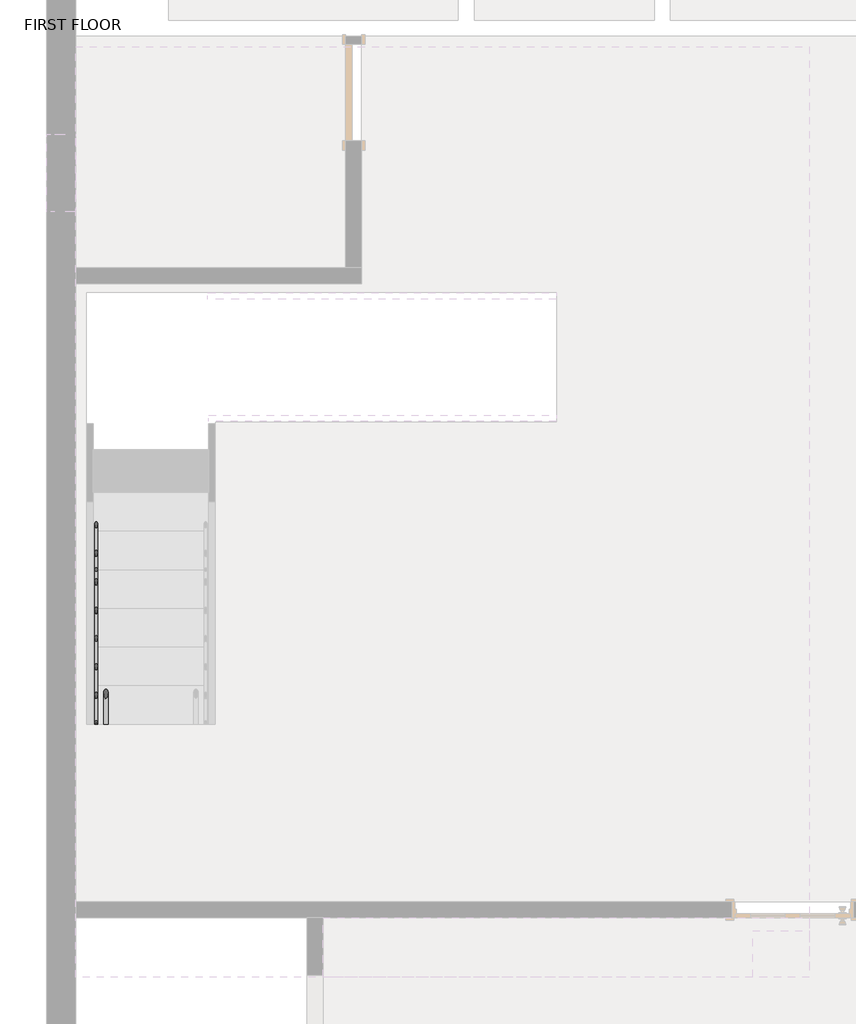
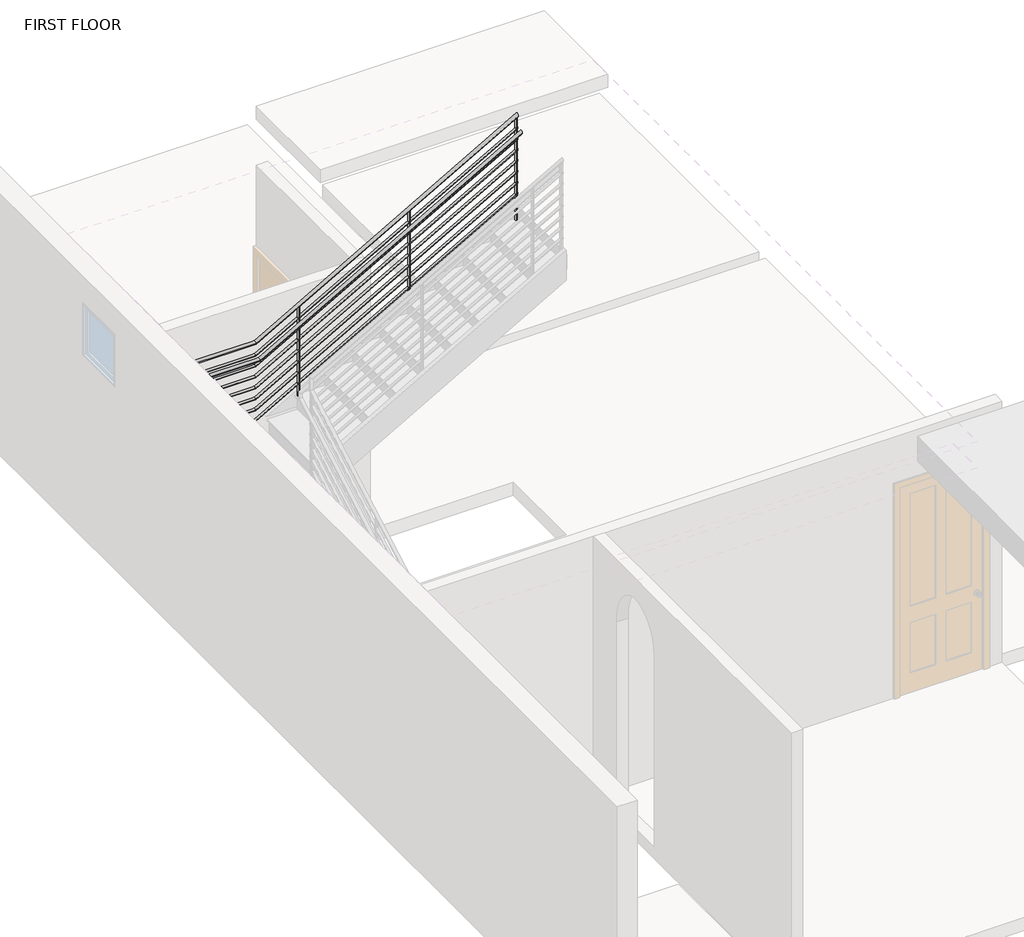
# One storey, part 2 of 3: 1 railing.
"""IFC4 building model written with IfcOpenShell, lengths in millimetres."""

from ifc_helpers import new_model, si_unit, point, frame, frame_2d, origin, place, context, project, spatial, circle_curve, ellipse_curve, trimmed, segment, composite_curve, outline, extrude, element, save
from ifc_brep_helpers import plane_surface, cylinder_surface, advanced_brep

model = new_model("IFC4")

# Units and contexts
model_context = context("Model", 3, world=origin())
ifc_project = project(units=[si_unit("LENGTHUNIT", "METRE", prefix="MILLI")], contexts=[model_context])

# Site, building, storey
site = spatial("IfcSite", under=ifc_project)
building = spatial("IfcBuilding", under=site)
storey = spatial("IfcBuildingStorey", under=building, Name="FIRST FLOOR", Elevation=3352.8)

# Railing
placement = place(None, origin())
element("IfcRailing", 1, ObjectType="Guardrail - Pipe", at=placement, inside=storey, context=model_context, shape_type="SolidModel", body=[
    advanced_brep(
    [(-6821.0257327, 1771.427543, 4418.0240066), (-6859.1257327, 1771.427543, 4418.0240066), (-6821.0257327, 4367.2498842, 5888.99), (-6859.1257327, 4367.2498842, 5888.99), (-6821.0257327, 5003.577543, 5888.99), (-6859.1257327, 5041.677543, 5888.99), (-6174.6533915, 5003.577543, 5888.99), (-6174.6533915, 5041.677543, 5888.99), (-3284.0757327, 5003.577543, 7526.9840066), (-3284.0757327, 5041.677543, 7526.9840066)],
    [
        (0, 1, ellipse_curve(frame((-6840.0757327, 1771.427543, 4418.0240066), z_axis=(0.0, -1.0, 0.0), x_axis=(0.0, 0.0, -1.0)), 21.8959934, 19.05)),
        (1, 0, ellipse_curve(frame((-6840.0757327, 1771.427543, 4418.0240066), z_axis=(0.0, -1.0, 0.0), x_axis=(0.0, 0.0, -1.0)), 21.8959934, 19.05)),
        (0, 2),
        (2, 3, ellipse_curve(frame((-6840.0757327, 4367.2498842, 5888.99), z_axis=(0.0, -0.9669597162882765, -0.25492921973696103), x_axis=(0.0, 0.25492921973696087, -0.9669597162882766)), 19.7009241, 19.05)),
        (3, 1),
        (3, 2, ellipse_curve(frame((-6840.0757327, 4367.2498842, 5888.99), z_axis=(0.0, -0.9669597162882765, -0.25492921973696103), x_axis=(0.0, 0.25492921973696087, -0.9669597162882766)), 19.7009241, 19.05)),
        (2, 4),
        (4, 5, ellipse_curve(frame((-6840.0757327, 5022.627543, 5888.99), z_axis=(-0.7071067811865486, -0.7071067811865465, 0.0), x_axis=(0.7071067811865465, -0.7071067811865486, 0.0)), 26.9407684, 19.05)),
        (5, 3),
        (5, 4, ellipse_curve(frame((-6840.0757327, 5022.627543, 5888.99), z_axis=(-0.7071067811865486, -0.7071067811865465, 0.0), x_axis=(0.7071067811865465, -0.7071067811865486, 0.0)), 26.9407684, 19.05)),
        (4, 6),
        (6, 7, ellipse_curve(frame((-6174.6533915, 5022.627543, 5888.99), z_axis=(-0.9669597162882765, 0.0, -0.254929219736961), x_axis=(-0.25492921973696137, 0.0, 0.9669597162882764)), 19.7009241, 19.05)),
        (7, 5),
        (7, 6, ellipse_curve(frame((-6174.6533915, 5022.627543, 5888.99), z_axis=(-0.9669597162882765, 0.0, -0.254929219736961), x_axis=(-0.25492921973696137, 0.0, 0.9669597162882764)), 19.7009241, 19.05)),
        (8, 9, ellipse_curve(frame((-3284.0757327, 5022.627543, 7526.9840066), z_axis=(1.0, 0.0, 0.0), x_axis=(0.0, 0.0, -0.9999999999999999)), 21.8959934, 19.05)),
        (9, 8, ellipse_curve(frame((-3284.0757327, 5022.627543, 7526.9840066), z_axis=(1.0, 0.0, 0.0), x_axis=(0.0, 0.0, -0.9999999999999999)), 21.8959934, 19.05)),
        (6, 8),
        (9, 7),
    ],
    [
        plane_surface(frame((-6840.0757327, 1771.427543, 4439.92), z_axis=(0.0, -1.0, 0.0), x_axis=(0.0, 0.0, 1.0))),
        cylinder_surface(frame((-6840.0757327, 1780.8194325, 4423.3460774), z_axis=(0.0, -0.8700221858486086, -0.4930125719808871), x_axis=(-1.0, 0.0, 0.0)), 19.05),
        cylinder_surface(frame((-6840.0757327, 4362.227543, 5888.99), z_axis=(0.0, -1.0, 0.0), x_axis=(-1.0, 0.0, 0.0)), 19.05),
        cylinder_surface(frame((-6840.0757327, 5022.627543, 5888.99), z_axis=(-1.0, 0.0, 0.0), x_axis=(0.0, 1.0, 0.0)), 19.05),
        plane_surface(frame((-3284.0757327, 5022.627543, 7548.88), z_axis=(1.0, 0.0, 0.0), x_axis=(0.0, 1.0, 0.0))),
        cylinder_surface(frame((-6170.2838432, 5022.627543, 5891.4660774), z_axis=(-0.8700221858486086, 0.0, -0.49301257198088694), x_axis=(0.0, 1.0, 0.0)), 19.05),
    ],
    [
        (0, [[1, 2]]),
        (1, [[-1, 3, 4, 5]]),
        (1, [[-2, -5, 6, -3]]),
        (2, [[-4, 7, 8, 9]]),
        (2, [[-6, -9, 10, -7]]),
        (3, [[-8, 11, 12, 13]]),
        (3, [[-10, -13, 14, -11]]),
        (4, [[15, 16]]),
        (5, [[-12, 17, -16, 18]]),
        (5, [[-14, -18, -15, -17]]),
    ],
),
    advanced_brep(
    [(-6897.2257327, 1771.427543, 4570.4240066), (-6935.3257327, 1771.427543, 4570.4240066), (-3284.0757327, 5079.777543, 7679.3840066), (-3284.0757327, 5117.877543, 7679.3840066), (-6897.2257327, 4367.2498842, 6041.39), (-6935.3257327, 4367.2498842, 6041.39), (-6897.2257327, 5079.777543, 6041.39), (-6935.3257327, 5117.877543, 6041.39), (-6174.6533915, 5079.777543, 6041.39), (-6174.6533915, 5117.877543, 6041.39)],
    [
        (0, 1, ellipse_curve(frame((-6916.2757327, 1771.427543, 4570.4240066), z_axis=(0.0, -1.0, 0.0), x_axis=(0.0, 0.0, -1.0)), 21.8959934, 19.05)),
        (1, 0, ellipse_curve(frame((-6916.2757327, 1771.427543, 4570.4240066), z_axis=(0.0, -1.0, 0.0), x_axis=(0.0, 0.0, -1.0)), 21.8959934, 19.05)),
        (2, 3, ellipse_curve(frame((-3284.0757327, 5098.827543, 7679.3840066), z_axis=(1.0, 0.0, 0.0), x_axis=(0.0, 0.0, -0.9999999999999999)), 21.8959934, 19.05)),
        (3, 2, ellipse_curve(frame((-3284.0757327, 5098.827543, 7679.3840066), z_axis=(1.0, 0.0, 0.0), x_axis=(0.0, 0.0, -0.9999999999999999)), 21.8959934, 19.05)),
        (0, 4),
        (4, 5, ellipse_curve(frame((-6916.2757327, 4367.2498842, 6041.39), z_axis=(0.0, -0.9669597162882765, -0.25492921973696103), x_axis=(0.0, 0.25492921973696087, -0.9669597162882766)), 19.7009241, 19.05)),
        (5, 1),
        (5, 4, ellipse_curve(frame((-6916.2757327, 4367.2498842, 6041.39), z_axis=(0.0, -0.9669597162882765, -0.25492921973696103), x_axis=(0.0, 0.25492921973696087, -0.9669597162882766)), 19.7009241, 19.05)),
        (4, 6),
        (6, 7, ellipse_curve(frame((-6916.2757327, 5098.827543, 6041.39), z_axis=(-0.7071067811865487, -0.7071067811865464, 0.0), x_axis=(0.7071067811865464, -0.7071067811865487, 0.0)), 26.9407684, 19.05)),
        (7, 5),
        (7, 6, ellipse_curve(frame((-6916.2757327, 5098.827543, 6041.39), z_axis=(-0.7071067811865487, -0.7071067811865464, 0.0), x_axis=(0.7071067811865464, -0.7071067811865487, 0.0)), 26.9407684, 19.05)),
        (6, 8),
        (8, 9, ellipse_curve(frame((-6174.6533915, 5098.827543, 6041.39), z_axis=(-0.9669597162882765, 0.0, -0.254929219736961), x_axis=(-0.25492921973696137, 0.0, 0.9669597162882764)), 19.7009241, 19.05)),
        (9, 7),
        (9, 8, ellipse_curve(frame((-6174.6533915, 5098.827543, 6041.39), z_axis=(-0.9669597162882765, 0.0, -0.254929219736961), x_axis=(-0.25492921973696137, 0.0, 0.9669597162882764)), 19.7009241, 19.05)),
        (8, 2),
        (3, 9),
    ],
    [
        plane_surface(frame((-6916.2757327, 1771.427543, 4592.32), z_axis=(0.0, -1.0, 0.0), x_axis=(0.0, 0.0, 1.0))),
        plane_surface(frame((-3284.0757327, 5098.827543, 7701.28), z_axis=(1.0, 0.0, 0.0), x_axis=(0.0, 1.0, 0.0))),
        cylinder_surface(frame((-6916.2757327, 1780.8194325, 4575.7460774), z_axis=(0.0, -0.8700221858486086, -0.4930125719808871), x_axis=(-1.0, 0.0, 0.0)), 19.05),
        cylinder_surface(frame((-6916.2757327, 4362.227543, 6041.39), z_axis=(0.0, -1.0, 0.0), x_axis=(-1.0, 0.0, 0.0)), 19.05),
        cylinder_surface(frame((-6916.2757327, 5098.827543, 6041.39), z_axis=(-1.0, 0.0, 0.0), x_axis=(0.0, 1.0, 0.0)), 19.05),
        cylinder_surface(frame((-6170.2838432, 5098.827543, 6043.8660774), z_axis=(-0.8700221858486086, 0.0, -0.49301257198088694), x_axis=(0.0, 1.0, 0.0)), 19.05),
    ],
    [
        (0, [[1, 2]]),
        (1, [[3, 4]]),
        (2, [[-1, 5, 6, 7]]),
        (2, [[-2, -7, 8, -5]]),
        (3, [[-6, 9, 10, 11]]),
        (3, [[-8, -11, 12, -9]]),
        (4, [[-10, 13, 14, 15]]),
        (4, [[-12, -15, 16, -13]]),
        (5, [[-14, 17, -4, 18]]),
        (5, [[-16, -18, -3, -17]]),
    ],
),
    advanced_brep(
    [(-6903.5757327, 1771.427543, 4425.3226711), (-6928.9757327, 1771.427543, 4425.3226711), (-6903.5757327, 4365.5757705, 5895.34), (-6928.9757327, 4365.5757705, 5895.34), (-6903.5757327, 5086.127543, 5895.34), (-6928.9757327, 5086.127543, 5895.34)],
    [
        (0, 1, ellipse_curve(frame((-6916.2757327, 1771.427543, 4425.3226711), z_axis=(0.0, -1.0, 0.0), x_axis=(0.0, 0.0, -1.0)), 14.5973289, 12.7)),
        (1, 0, ellipse_curve(frame((-6916.2757327, 1771.427543, 4425.3226711), z_axis=(0.0, -1.0, 0.0), x_axis=(0.0, 0.0, -1.0)), 14.5973289, 12.7)),
        (0, 2),
        (2, 3, ellipse_curve(frame((-6916.2757327, 4365.5757705, 5895.34), z_axis=(0.0, -0.9669597162882765, -0.25492921973696103), x_axis=(0.0, 0.25492921973696087, -0.9669597162882766)), 13.1339494, 12.7)),
        (3, 1),
        (3, 2, ellipse_curve(frame((-6916.2757327, 4365.5757705, 5895.34), z_axis=(0.0, -0.9669597162882765, -0.25492921973696103), x_axis=(0.0, 0.25492921973696087, -0.9669597162882766)), 13.1339494, 12.7)),
        (4, 5, circle_curve(frame((-6916.2757327, 5086.127543, 5895.34), z_axis=(0.0, 1.0, 0.0), x_axis=(-1.0, 0.0, 0.0)), 12.7)),
        (5, 4, circle_curve(frame((-6916.2757327, 5086.127543, 5895.34), z_axis=(0.0, 1.0, 0.0), x_axis=(-1.0, 0.0, 0.0)), 12.7)),
        (2, 4),
        (5, 3),
    ],
    [
        plane_surface(frame((-6916.2757327, 1771.427543, 4439.92), z_axis=(0.0, -1.0, 0.0), x_axis=(0.0, 0.0, 1.0))),
        cylinder_surface(frame((-6916.2757327, 1777.6888026, 4428.8707182), z_axis=(0.0, -0.8700221858486086, -0.4930125719808871), x_axis=(-1.0, 0.0, 0.0)), 12.7),
        plane_surface(frame((-6916.2757327, 5086.127543, 5908.04), z_axis=(0.0, 1.0, 0.0), x_axis=(0.0, 0.0, 1.0))),
        cylinder_surface(frame((-6916.2757327, 4362.227543, 5895.34), z_axis=(0.0, -1.0, 0.0), x_axis=(-1.0, 0.0, 0.0)), 12.7),
    ],
    [
        (0, [[1, 2]]),
        (1, [[-1, 3, 4, 5]]),
        (1, [[-2, -5, 6, -3]]),
        (2, [[7, 8]]),
        (3, [[-4, 9, -8, 10]]),
        (3, [[-6, -10, -7, -9]]),
    ],
),
    advanced_brep(
    [(-6928.9757327, 5086.127543, 5895.34), (-6928.9757327, 5111.527543, 5895.34), (-6176.3275052, 5086.127543, 5895.34), (-6176.3275052, 5111.527543, 5895.34), (-3284.0757327, 5086.127543, 7534.2826711), (-3284.0757327, 5111.527543, 7534.2826711)],
    [
        (0, 1, circle_curve(frame((-6928.9757327, 5098.827543, 5895.34), z_axis=(-1.0, 0.0, 0.0), x_axis=(0.0, 1.0, 0.0)), 12.7)),
        (1, 0, circle_curve(frame((-6928.9757327, 5098.827543, 5895.34), z_axis=(-1.0, 0.0, 0.0), x_axis=(0.0, 1.0, 0.0)), 12.7)),
        (0, 2),
        (2, 3, ellipse_curve(frame((-6176.3275052, 5098.827543, 5895.34), z_axis=(-0.9669597162882765, 0.0, -0.2549292197369609), x_axis=(-0.25492921973696137, 0.0, 0.9669597162882764)), 13.1339494, 12.7)),
        (3, 1),
        (3, 2, ellipse_curve(frame((-6176.3275052, 5098.827543, 5895.34), z_axis=(-0.9669597162882765, 0.0, -0.2549292197369609), x_axis=(-0.25492921973696137, 0.0, 0.9669597162882764)), 13.1339494, 12.7)),
        (4, 5, ellipse_curve(frame((-3284.0757327, 5098.827543, 7534.2826711), z_axis=(1.0, 0.0, 0.0), x_axis=(0.0, 0.0, -0.9999999999999999)), 14.5973289, 12.7)),
        (5, 4, ellipse_curve(frame((-3284.0757327, 5098.827543, 7534.2826711), z_axis=(1.0, 0.0, 0.0), x_axis=(0.0, 0.0, -0.9999999999999999)), 14.5973289, 12.7)),
        (2, 4),
        (5, 3),
    ],
    [
        plane_surface(frame((-6928.9757327, 5098.827543, 5908.04), z_axis=(-1.0, 0.0, 0.0), x_axis=(0.0, 1.0, 0.0))),
        cylinder_surface(frame((-6928.9757327, 5098.827543, 5895.34), z_axis=(-1.0, 0.0, 0.0), x_axis=(0.0, 1.0, 0.0)), 12.7),
        plane_surface(frame((-3284.0757327, 5098.827543, 7548.88), z_axis=(1.0, 0.0, 0.0), x_axis=(0.0, 1.0, 0.0))),
        cylinder_surface(frame((-6173.414473, 5098.827543, 5896.9907182), z_axis=(-0.8700221858486087, 0.0, -0.49301257198088694), x_axis=(0.0, 1.0, 0.0)), 12.7),
    ],
    [
        (0, [[1, 2]]),
        (1, [[-1, 3, 4, 5]]),
        (1, [[-2, -5, 6, -3]]),
        (2, [[7, 8]]),
        (3, [[-4, 9, -8, 10]]),
        (3, [[-6, -10, -7, -9]]),
    ],
),
    advanced_brep(
    [(-6903.5757327, 1771.427543, 4298.3226711), (-6928.9757327, 1771.427543, 4298.3226711), (-6903.5757327, 4365.5757705, 5768.34), (-6928.9757327, 4365.5757705, 5768.34), (-6903.5757327, 5086.127543, 5768.34), (-6928.9757327, 5086.127543, 5768.34)],
    [
        (0, 1, ellipse_curve(frame((-6916.2757327, 1771.427543, 4298.3226711), z_axis=(0.0, -1.0, 0.0), x_axis=(0.0, 0.0, -1.0)), 14.5973289, 12.7)),
        (1, 0, ellipse_curve(frame((-6916.2757327, 1771.427543, 4298.3226711), z_axis=(0.0, -1.0, 0.0), x_axis=(0.0, 0.0, -1.0)), 14.5973289, 12.7)),
        (0, 2),
        (2, 3, ellipse_curve(frame((-6916.2757327, 4365.5757705, 5768.34), z_axis=(0.0, -0.9669597162882765, -0.25492921973696103), x_axis=(0.0, 0.25492921973696087, -0.9669597162882766)), 13.1339494, 12.7)),
        (3, 1),
        (3, 2, ellipse_curve(frame((-6916.2757327, 4365.5757705, 5768.34), z_axis=(0.0, -0.9669597162882765, -0.25492921973696103), x_axis=(0.0, 0.25492921973696087, -0.9669597162882766)), 13.1339494, 12.7)),
        (4, 5, circle_curve(frame((-6916.2757327, 5086.127543, 5768.34), z_axis=(0.0, 1.0, 0.0), x_axis=(-1.0, 0.0, 0.0)), 12.7)),
        (5, 4, circle_curve(frame((-6916.2757327, 5086.127543, 5768.34), z_axis=(0.0, 1.0, 0.0), x_axis=(-1.0, 0.0, 0.0)), 12.7)),
        (2, 4),
        (5, 3),
    ],
    [
        plane_surface(frame((-6916.2757327, 1771.427543, 4312.92), z_axis=(0.0, -1.0, 0.0), x_axis=(0.0, 0.0, 1.0))),
        cylinder_surface(frame((-6916.2757327, 1777.6888026, 4301.8707182), z_axis=(0.0, -0.8700221858486086, -0.4930125719808871), x_axis=(-1.0, 0.0, 0.0)), 12.7),
        plane_surface(frame((-6916.2757327, 5086.127543, 5781.04), z_axis=(0.0, 1.0, 0.0), x_axis=(0.0, 0.0, 1.0))),
        cylinder_surface(frame((-6916.2757327, 4362.227543, 5768.34), z_axis=(0.0, -1.0, 0.0), x_axis=(-1.0, 0.0, 0.0)), 12.7),
    ],
    [
        (0, [[1, 2]]),
        (1, [[-1, 3, 4, 5]]),
        (1, [[-2, -5, 6, -3]]),
        (2, [[7, 8]]),
        (3, [[-4, 9, -8, 10]]),
        (3, [[-6, -10, -7, -9]]),
    ],
),
    advanced_brep(
    [(-6928.9757327, 5086.127543, 5768.34), (-6928.9757327, 5111.527543, 5768.34), (-6176.3275052, 5086.127543, 5768.34), (-6176.3275052, 5111.527543, 5768.34), (-3284.0757327, 5086.127543, 7407.2826711), (-3284.0757327, 5111.527543, 7407.2826711)],
    [
        (0, 1, circle_curve(frame((-6928.9757327, 5098.827543, 5768.34), z_axis=(-1.0, 0.0, 0.0), x_axis=(0.0, 1.0, 0.0)), 12.7)),
        (1, 0, circle_curve(frame((-6928.9757327, 5098.827543, 5768.34), z_axis=(-1.0, 0.0, 0.0), x_axis=(0.0, 1.0, 0.0)), 12.7)),
        (0, 2),
        (2, 3, ellipse_curve(frame((-6176.3275052, 5098.827543, 5768.34), z_axis=(-0.9669597162882765, 0.0, -0.2549292197369609), x_axis=(-0.25492921973696137, 0.0, 0.9669597162882764)), 13.1339494, 12.7)),
        (3, 1),
        (3, 2, ellipse_curve(frame((-6176.3275052, 5098.827543, 5768.34), z_axis=(-0.9669597162882765, 0.0, -0.2549292197369609), x_axis=(-0.25492921973696137, 0.0, 0.9669597162882764)), 13.1339494, 12.7)),
        (4, 5, ellipse_curve(frame((-3284.0757327, 5098.827543, 7407.2826711), z_axis=(1.0, 0.0, 0.0), x_axis=(0.0, 0.0, -0.9999999999999999)), 14.5973289, 12.7)),
        (5, 4, ellipse_curve(frame((-3284.0757327, 5098.827543, 7407.2826711), z_axis=(1.0, 0.0, 0.0), x_axis=(0.0, 0.0, -0.9999999999999999)), 14.5973289, 12.7)),
        (2, 4),
        (5, 3),
    ],
    [
        plane_surface(frame((-6928.9757327, 5098.827543, 5781.04), z_axis=(-1.0, 0.0, 0.0), x_axis=(0.0, 1.0, 0.0))),
        cylinder_surface(frame((-6928.9757327, 5098.827543, 5768.34), z_axis=(-1.0, 0.0, 0.0), x_axis=(0.0, 1.0, 0.0)), 12.7),
        plane_surface(frame((-3284.0757327, 5098.827543, 7421.88), z_axis=(1.0, 0.0, 0.0), x_axis=(0.0, 1.0, 0.0))),
        cylinder_surface(frame((-6173.414473, 5098.827543, 5769.9907182), z_axis=(-0.8700221858486087, 0.0, -0.49301257198088694), x_axis=(0.0, 1.0, 0.0)), 12.7),
    ],
    [
        (0, [[1, 2]]),
        (1, [[-1, 3, 4, 5]]),
        (1, [[-2, -5, 6, -3]]),
        (2, [[7, 8]]),
        (3, [[-4, 9, -8, 10]]),
        (3, [[-6, -10, -7, -9]]),
    ],
),
    advanced_brep(
    [(-6903.5757327, 1771.427543, 4171.3226711), (-6928.9757327, 1771.427543, 4171.3226711), (-6903.5757327, 4365.5757705, 5641.34), (-6928.9757327, 4365.5757705, 5641.34), (-6903.5757327, 5086.127543, 5641.34), (-6928.9757327, 5086.127543, 5641.34)],
    [
        (0, 1, ellipse_curve(frame((-6916.2757327, 1771.427543, 4171.3226711), z_axis=(0.0, -1.0, 0.0), x_axis=(0.0, 0.0, -1.0)), 14.5973289, 12.7)),
        (1, 0, ellipse_curve(frame((-6916.2757327, 1771.427543, 4171.3226711), z_axis=(0.0, -1.0, 0.0), x_axis=(0.0, 0.0, -1.0)), 14.5973289, 12.7)),
        (0, 2),
        (2, 3, ellipse_curve(frame((-6916.2757327, 4365.5757705, 5641.34), z_axis=(0.0, -0.9669597162882765, -0.25492921973696103), x_axis=(0.0, 0.25492921973696087, -0.9669597162882766)), 13.1339494, 12.7)),
        (3, 1),
        (3, 2, ellipse_curve(frame((-6916.2757327, 4365.5757705, 5641.34), z_axis=(0.0, -0.9669597162882765, -0.25492921973696103), x_axis=(0.0, 0.25492921973696087, -0.9669597162882766)), 13.1339494, 12.7)),
        (4, 5, circle_curve(frame((-6916.2757327, 5086.127543, 5641.34), z_axis=(0.0, 1.0, 0.0), x_axis=(-1.0, 0.0, 0.0)), 12.7)),
        (5, 4, circle_curve(frame((-6916.2757327, 5086.127543, 5641.34), z_axis=(0.0, 1.0, 0.0), x_axis=(-1.0, 0.0, 0.0)), 12.7)),
        (2, 4),
        (5, 3),
    ],
    [
        plane_surface(frame((-6916.2757327, 1771.427543, 4185.92), z_axis=(0.0, -1.0, 0.0), x_axis=(0.0, 0.0, 1.0))),
        cylinder_surface(frame((-6916.2757327, 1777.6888026, 4174.8707182), z_axis=(0.0, -0.8700221858486086, -0.4930125719808871), x_axis=(-1.0, 0.0, 0.0)), 12.7),
        plane_surface(frame((-6916.2757327, 5086.127543, 5654.04), z_axis=(0.0, 1.0, 0.0), x_axis=(0.0, 0.0, 1.0))),
        cylinder_surface(frame((-6916.2757327, 4362.227543, 5641.34), z_axis=(0.0, -1.0, 0.0), x_axis=(-1.0, 0.0, 0.0)), 12.7),
    ],
    [
        (0, [[1, 2]]),
        (1, [[-1, 3, 4, 5]]),
        (1, [[-2, -5, 6, -3]]),
        (2, [[7, 8]]),
        (3, [[-4, 9, -8, 10]]),
        (3, [[-6, -10, -7, -9]]),
    ],
),
    advanced_brep(
    [(-6928.9757327, 5086.127543, 5641.34), (-6928.9757327, 5111.527543, 5641.34), (-6176.3275052, 5086.127543, 5641.34), (-6176.3275052, 5111.527543, 5641.34), (-3284.0757327, 5086.127543, 7280.2826711), (-3284.0757327, 5111.527543, 7280.2826711)],
    [
        (0, 1, circle_curve(frame((-6928.9757327, 5098.827543, 5641.34), z_axis=(-1.0, 0.0, 0.0), x_axis=(0.0, 1.0, 0.0)), 12.7)),
        (1, 0, circle_curve(frame((-6928.9757327, 5098.827543, 5641.34), z_axis=(-1.0, 0.0, 0.0), x_axis=(0.0, 1.0, 0.0)), 12.7)),
        (0, 2),
        (2, 3, ellipse_curve(frame((-6176.3275052, 5098.827543, 5641.34), z_axis=(-0.9669597162882765, 0.0, -0.2549292197369609), x_axis=(-0.25492921973696137, 0.0, 0.9669597162882764)), 13.1339494, 12.7)),
        (3, 1),
        (3, 2, ellipse_curve(frame((-6176.3275052, 5098.827543, 5641.34), z_axis=(-0.9669597162882765, 0.0, -0.2549292197369609), x_axis=(-0.25492921973696137, 0.0, 0.9669597162882764)), 13.1339494, 12.7)),
        (4, 5, ellipse_curve(frame((-3284.0757327, 5098.827543, 7280.2826711), z_axis=(1.0, 0.0, 0.0), x_axis=(0.0, 0.0, -0.9999999999999999)), 14.5973289, 12.7)),
        (5, 4, ellipse_curve(frame((-3284.0757327, 5098.827543, 7280.2826711), z_axis=(1.0, 0.0, 0.0), x_axis=(0.0, 0.0, -0.9999999999999999)), 14.5973289, 12.7)),
        (2, 4),
        (5, 3),
    ],
    [
        plane_surface(frame((-6928.9757327, 5098.827543, 5654.04), z_axis=(-1.0, 0.0, 0.0), x_axis=(0.0, 1.0, 0.0))),
        cylinder_surface(frame((-6928.9757327, 5098.827543, 5641.34), z_axis=(-1.0, 0.0, 0.0), x_axis=(0.0, 1.0, 0.0)), 12.7),
        plane_surface(frame((-3284.0757327, 5098.827543, 7294.88), z_axis=(1.0, 0.0, 0.0), x_axis=(0.0, 1.0, 0.0))),
        cylinder_surface(frame((-6173.414473, 5098.827543, 5642.9907182), z_axis=(-0.8700221858486087, 0.0, -0.49301257198088694), x_axis=(0.0, 1.0, 0.0)), 12.7),
    ],
    [
        (0, [[1, 2]]),
        (1, [[-1, 3, 4, 5]]),
        (1, [[-2, -5, 6, -3]]),
        (2, [[7, 8]]),
        (3, [[-4, 9, -8, 10]]),
        (3, [[-6, -10, -7, -9]]),
    ],
),
    advanced_brep(
    [(-6903.5757327, 1771.427543, 4044.3226711), (-6928.9757327, 1771.427543, 4044.3226711), (-6903.5757327, 4365.5757705, 5514.34), (-6928.9757327, 4365.5757705, 5514.34), (-6903.5757327, 5086.127543, 5514.34), (-6928.9757327, 5086.127543, 5514.34)],
    [
        (0, 1, ellipse_curve(frame((-6916.2757327, 1771.427543, 4044.3226711), z_axis=(0.0, -1.0, 0.0), x_axis=(0.0, 0.0, -1.0)), 14.5973289, 12.7)),
        (1, 0, ellipse_curve(frame((-6916.2757327, 1771.427543, 4044.3226711), z_axis=(0.0, -1.0, 0.0), x_axis=(0.0, 0.0, -1.0)), 14.5973289, 12.7)),
        (0, 2),
        (2, 3, ellipse_curve(frame((-6916.2757327, 4365.5757705, 5514.34), z_axis=(0.0, -0.9669597162882765, -0.25492921973696103), x_axis=(0.0, 0.25492921973696087, -0.9669597162882766)), 13.1339494, 12.7)),
        (3, 1),
        (3, 2, ellipse_curve(frame((-6916.2757327, 4365.5757705, 5514.34), z_axis=(0.0, -0.9669597162882765, -0.25492921973696103), x_axis=(0.0, 0.25492921973696087, -0.9669597162882766)), 13.1339494, 12.7)),
        (4, 5, circle_curve(frame((-6916.2757327, 5086.127543, 5514.34), z_axis=(0.0, 1.0, 0.0), x_axis=(-1.0, 0.0, 0.0)), 12.7)),
        (5, 4, circle_curve(frame((-6916.2757327, 5086.127543, 5514.34), z_axis=(0.0, 1.0, 0.0), x_axis=(-1.0, 0.0, 0.0)), 12.7)),
        (2, 4),
        (5, 3),
    ],
    [
        plane_surface(frame((-6916.2757327, 1771.427543, 4058.92), z_axis=(0.0, -1.0, 0.0), x_axis=(0.0, 0.0, 1.0))),
        cylinder_surface(frame((-6916.2757327, 1777.6888026, 4047.8707182), z_axis=(0.0, -0.8700221858486086, -0.4930125719808871), x_axis=(-1.0, 0.0, 0.0)), 12.7),
        plane_surface(frame((-6916.2757327, 5086.127543, 5527.04), z_axis=(0.0, 1.0, 0.0), x_axis=(0.0, 0.0, 1.0))),
        cylinder_surface(frame((-6916.2757327, 4362.227543, 5514.34), z_axis=(0.0, -1.0, 0.0), x_axis=(-1.0, 0.0, 0.0)), 12.7),
    ],
    [
        (0, [[1, 2]]),
        (1, [[-1, 3, 4, 5]]),
        (1, [[-2, -5, 6, -3]]),
        (2, [[7, 8]]),
        (3, [[-4, 9, -8, 10]]),
        (3, [[-6, -10, -7, -9]]),
    ],
),
    advanced_brep(
    [(-6928.9757327, 5086.127543, 5514.34), (-6928.9757327, 5111.527543, 5514.34), (-6176.3275052, 5086.127543, 5514.34), (-6176.3275052, 5111.527543, 5514.34), (-3284.0757327, 5086.127543, 7153.2826711), (-3284.0757327, 5111.527543, 7153.2826711)],
    [
        (0, 1, circle_curve(frame((-6928.9757327, 5098.827543, 5514.34), z_axis=(-1.0, 0.0, 0.0), x_axis=(0.0, 1.0, 0.0)), 12.7)),
        (1, 0, circle_curve(frame((-6928.9757327, 5098.827543, 5514.34), z_axis=(-1.0, 0.0, 0.0), x_axis=(0.0, 1.0, 0.0)), 12.7)),
        (0, 2),
        (2, 3, ellipse_curve(frame((-6176.3275052, 5098.827543, 5514.34), z_axis=(-0.9669597162882765, 0.0, -0.2549292197369609), x_axis=(-0.25492921973696137, 0.0, 0.9669597162882764)), 13.1339494, 12.7)),
        (3, 1),
        (3, 2, ellipse_curve(frame((-6176.3275052, 5098.827543, 5514.34), z_axis=(-0.9669597162882765, 0.0, -0.2549292197369609), x_axis=(-0.25492921973696137, 0.0, 0.9669597162882764)), 13.1339494, 12.7)),
        (4, 5, ellipse_curve(frame((-3284.0757327, 5098.827543, 7153.2826711), z_axis=(1.0, 0.0, 0.0), x_axis=(0.0, 0.0, -0.9999999999999999)), 14.5973289, 12.7)),
        (5, 4, ellipse_curve(frame((-3284.0757327, 5098.827543, 7153.2826711), z_axis=(1.0, 0.0, 0.0), x_axis=(0.0, 0.0, -0.9999999999999999)), 14.5973289, 12.7)),
        (2, 4),
        (5, 3),
    ],
    [
        plane_surface(frame((-6928.9757327, 5098.827543, 5527.04), z_axis=(-1.0, 0.0, 0.0), x_axis=(0.0, 1.0, 0.0))),
        cylinder_surface(frame((-6928.9757327, 5098.827543, 5514.34), z_axis=(-1.0, 0.0, 0.0), x_axis=(0.0, 1.0, 0.0)), 12.7),
        plane_surface(frame((-3284.0757327, 5098.827543, 7167.88), z_axis=(1.0, 0.0, 0.0), x_axis=(0.0, 1.0, 0.0))),
        cylinder_surface(frame((-6173.414473, 5098.827543, 5515.9907182), z_axis=(-0.8700221858486087, 0.0, -0.49301257198088694), x_axis=(0.0, 1.0, 0.0)), 12.7),
    ],
    [
        (0, [[1, 2]]),
        (1, [[-1, 3, 4, 5]]),
        (1, [[-2, -5, 6, -3]]),
        (2, [[7, 8]]),
        (3, [[-4, 9, -8, 10]]),
        (3, [[-6, -10, -7, -9]]),
    ],
),
    advanced_brep(
    [(-6903.5757327, 1771.427543, 3917.3226711), (-6928.9757327, 1771.427543, 3917.3226711), (-6903.5757327, 4365.5757705, 5387.34), (-6928.9757327, 4365.5757705, 5387.34), (-6903.5757327, 5086.127543, 5387.34), (-6928.9757327, 5086.127543, 5387.34)],
    [
        (0, 1, ellipse_curve(frame((-6916.2757327, 1771.427543, 3917.3226711), z_axis=(0.0, -1.0, 0.0), x_axis=(0.0, 0.0, -1.0)), 14.5973289, 12.7)),
        (1, 0, ellipse_curve(frame((-6916.2757327, 1771.427543, 3917.3226711), z_axis=(0.0, -1.0, 0.0), x_axis=(0.0, 0.0, -1.0)), 14.5973289, 12.7)),
        (0, 2),
        (2, 3, ellipse_curve(frame((-6916.2757327, 4365.5757705, 5387.34), z_axis=(0.0, -0.9669597162882765, -0.25492921973696103), x_axis=(0.0, 0.25492921973696087, -0.9669597162882766)), 13.1339494, 12.7)),
        (3, 1),
        (3, 2, ellipse_curve(frame((-6916.2757327, 4365.5757705, 5387.34), z_axis=(0.0, -0.9669597162882765, -0.25492921973696103), x_axis=(0.0, 0.25492921973696087, -0.9669597162882766)), 13.1339494, 12.7)),
        (4, 5, circle_curve(frame((-6916.2757327, 5086.127543, 5387.34), z_axis=(0.0, 1.0, 0.0), x_axis=(-1.0, 0.0, 0.0)), 12.7)),
        (5, 4, circle_curve(frame((-6916.2757327, 5086.127543, 5387.34), z_axis=(0.0, 1.0, 0.0), x_axis=(-1.0, 0.0, 0.0)), 12.7)),
        (2, 4),
        (5, 3),
    ],
    [
        plane_surface(frame((-6916.2757327, 1771.427543, 3931.92), z_axis=(0.0, -1.0, 0.0), x_axis=(0.0, 0.0, 1.0))),
        cylinder_surface(frame((-6916.2757327, 1777.6888026, 3920.8707182), z_axis=(0.0, -0.8700221858486086, -0.4930125719808871), x_axis=(-1.0, 0.0, 0.0)), 12.7),
        plane_surface(frame((-6916.2757327, 5086.127543, 5400.04), z_axis=(0.0, 1.0, 0.0), x_axis=(0.0, 0.0, 1.0))),
        cylinder_surface(frame((-6916.2757327, 4362.227543, 5387.34), z_axis=(0.0, -1.0, 0.0), x_axis=(-1.0, 0.0, 0.0)), 12.7),
    ],
    [
        (0, [[1, 2]]),
        (1, [[-1, 3, 4, 5]]),
        (1, [[-2, -5, 6, -3]]),
        (2, [[7, 8]]),
        (3, [[-4, 9, -8, 10]]),
        (3, [[-6, -10, -7, -9]]),
    ],
),
    advanced_brep(
    [(-6928.9757327, 5086.127543, 5387.34), (-6928.9757327, 5111.527543, 5387.34), (-6176.3275052, 5086.127543, 5387.34), (-6176.3275052, 5111.527543, 5387.34), (-3284.0757327, 5086.127543, 7026.2826711), (-3284.0757327, 5111.527543, 7026.2826711)],
    [
        (0, 1, circle_curve(frame((-6928.9757327, 5098.827543, 5387.34), z_axis=(-1.0, 0.0, 0.0), x_axis=(0.0, 1.0, 0.0)), 12.7)),
        (1, 0, circle_curve(frame((-6928.9757327, 5098.827543, 5387.34), z_axis=(-1.0, 0.0, 0.0), x_axis=(0.0, 1.0, 0.0)), 12.7)),
        (0, 2),
        (2, 3, ellipse_curve(frame((-6176.3275052, 5098.827543, 5387.34), z_axis=(-0.9669597162882765, 0.0, -0.2549292197369609), x_axis=(-0.25492921973696137, 0.0, 0.9669597162882764)), 13.1339494, 12.7)),
        (3, 1),
        (3, 2, ellipse_curve(frame((-6176.3275052, 5098.827543, 5387.34), z_axis=(-0.9669597162882765, 0.0, -0.2549292197369609), x_axis=(-0.25492921973696137, 0.0, 0.9669597162882764)), 13.1339494, 12.7)),
        (4, 5, ellipse_curve(frame((-3284.0757327, 5098.827543, 7026.2826711), z_axis=(1.0, 0.0, 0.0), x_axis=(0.0, 0.0, -0.9999999999999999)), 14.5973289, 12.7)),
        (5, 4, ellipse_curve(frame((-3284.0757327, 5098.827543, 7026.2826711), z_axis=(1.0, 0.0, 0.0), x_axis=(0.0, 0.0, -0.9999999999999999)), 14.5973289, 12.7)),
        (2, 4),
        (5, 3),
    ],
    [
        plane_surface(frame((-6928.9757327, 5098.827543, 5400.04), z_axis=(-1.0, 0.0, 0.0), x_axis=(0.0, 1.0, 0.0))),
        cylinder_surface(frame((-6928.9757327, 5098.827543, 5387.34), z_axis=(-1.0, 0.0, 0.0), x_axis=(0.0, 1.0, 0.0)), 12.7),
        plane_surface(frame((-3284.0757327, 5098.827543, 7040.88), z_axis=(1.0, 0.0, 0.0), x_axis=(0.0, 1.0, 0.0))),
        cylinder_surface(frame((-6173.414473, 5098.827543, 5388.9907182), z_axis=(-0.8700221858486087, 0.0, -0.49301257198088694), x_axis=(0.0, 1.0, 0.0)), 12.7),
    ],
    [
        (0, [[1, 2]]),
        (1, [[-1, 3, 4, 5]]),
        (1, [[-2, -5, 6, -3]]),
        (2, [[7, 8]]),
        (3, [[-4, 9, -8, 10]]),
        (3, [[-6, -10, -7, -9]]),
    ],
),
    advanced_brep(
    [(-6903.5757327, 1771.427543, 3790.3226711), (-6928.9757327, 1771.427543, 3790.3226711), (-6903.5757327, 4365.5757705, 5260.34), (-6928.9757327, 4365.5757705, 5260.34), (-6903.5757327, 5086.127543, 5260.34), (-6928.9757327, 5086.127543, 5260.34)],
    [
        (0, 1, ellipse_curve(frame((-6916.2757327, 1771.427543, 3790.3226711), z_axis=(0.0, -1.0, 0.0), x_axis=(0.0, 0.0, -1.0)), 14.5973289, 12.7)),
        (1, 0, ellipse_curve(frame((-6916.2757327, 1771.427543, 3790.3226711), z_axis=(0.0, -1.0, 0.0), x_axis=(0.0, 0.0, -1.0)), 14.5973289, 12.7)),
        (0, 2),
        (2, 3, ellipse_curve(frame((-6916.2757327, 4365.5757705, 5260.34), z_axis=(0.0, -0.9669597162882765, -0.25492921973696103), x_axis=(0.0, 0.25492921973696087, -0.9669597162882766)), 13.1339494, 12.7)),
        (3, 1),
        (3, 2, ellipse_curve(frame((-6916.2757327, 4365.5757705, 5260.34), z_axis=(0.0, -0.9669597162882765, -0.25492921973696103), x_axis=(0.0, 0.25492921973696087, -0.9669597162882766)), 13.1339494, 12.7)),
        (4, 5, circle_curve(frame((-6916.2757327, 5086.127543, 5260.34), z_axis=(0.0, 1.0, 0.0), x_axis=(-1.0, 0.0, 0.0)), 12.7)),
        (5, 4, circle_curve(frame((-6916.2757327, 5086.127543, 5260.34), z_axis=(0.0, 1.0, 0.0), x_axis=(-1.0, 0.0, 0.0)), 12.7)),
        (2, 4),
        (5, 3),
    ],
    [
        plane_surface(frame((-6916.2757327, 1771.427543, 3804.92), z_axis=(0.0, -1.0, 0.0), x_axis=(0.0, 0.0, 1.0))),
        cylinder_surface(frame((-6916.2757327, 1777.6888026, 3793.8707182), z_axis=(0.0, -0.8700221858486086, -0.4930125719808871), x_axis=(-1.0, 0.0, 0.0)), 12.7),
        plane_surface(frame((-6916.2757327, 5086.127543, 5273.04), z_axis=(0.0, 1.0, 0.0), x_axis=(0.0, 0.0, 1.0))),
        cylinder_surface(frame((-6916.2757327, 4362.227543, 5260.34), z_axis=(0.0, -1.0, 0.0), x_axis=(-1.0, 0.0, 0.0)), 12.7),
    ],
    [
        (0, [[1, 2]]),
        (1, [[-1, 3, 4, 5]]),
        (1, [[-2, -5, 6, -3]]),
        (2, [[7, 8]]),
        (3, [[-4, 9, -8, 10]]),
        (3, [[-6, -10, -7, -9]]),
    ],
),
    advanced_brep(
    [(-6928.9757327, 5086.127543, 5260.34), (-6928.9757327, 5111.527543, 5260.34), (-6176.3275052, 5086.127543, 5260.34), (-6176.3275052, 5111.527543, 5260.34), (-3284.0757327, 5086.127543, 6899.2826711), (-3284.0757327, 5111.527543, 6899.2826711)],
    [
        (0, 1, circle_curve(frame((-6928.9757327, 5098.827543, 5260.34), z_axis=(-1.0, 0.0, 0.0), x_axis=(0.0, 1.0, 0.0)), 12.7)),
        (1, 0, circle_curve(frame((-6928.9757327, 5098.827543, 5260.34), z_axis=(-1.0, 0.0, 0.0), x_axis=(0.0, 1.0, 0.0)), 12.7)),
        (0, 2),
        (2, 3, ellipse_curve(frame((-6176.3275052, 5098.827543, 5260.34), z_axis=(-0.9669597162882765, 0.0, -0.2549292197369609), x_axis=(-0.25492921973696137, 0.0, 0.9669597162882764)), 13.1339494, 12.7)),
        (3, 1),
        (3, 2, ellipse_curve(frame((-6176.3275052, 5098.827543, 5260.34), z_axis=(-0.9669597162882765, 0.0, -0.2549292197369609), x_axis=(-0.25492921973696137, 0.0, 0.9669597162882764)), 13.1339494, 12.7)),
        (4, 5, ellipse_curve(frame((-3284.0757327, 5098.827543, 6899.2826711), z_axis=(1.0, 0.0, 0.0), x_axis=(0.0, 0.0, -0.9999999999999999)), 14.5973289, 12.7)),
        (5, 4, ellipse_curve(frame((-3284.0757327, 5098.827543, 6899.2826711), z_axis=(1.0, 0.0, 0.0), x_axis=(0.0, 0.0, -0.9999999999999999)), 14.5973289, 12.7)),
        (2, 4),
        (5, 3),
    ],
    [
        plane_surface(frame((-6928.9757327, 5098.827543, 5273.04), z_axis=(-1.0, 0.0, 0.0), x_axis=(0.0, 1.0, 0.0))),
        cylinder_surface(frame((-6928.9757327, 5098.827543, 5260.34), z_axis=(-1.0, 0.0, 0.0), x_axis=(0.0, 1.0, 0.0)), 12.7),
        plane_surface(frame((-3284.0757327, 5098.827543, 6913.88), z_axis=(1.0, 0.0, 0.0), x_axis=(0.0, 1.0, 0.0))),
        cylinder_surface(frame((-6173.414473, 5098.827543, 5261.9907182), z_axis=(-0.8700221858486087, 0.0, -0.49301257198088694), x_axis=(0.0, 1.0, 0.0)), 12.7),
    ],
    [
        (0, [[1, 2]]),
        (1, [[-1, 3, 4, 5]]),
        (1, [[-2, -5, 6, -3]]),
        (2, [[7, 8]]),
        (3, [[-4, 9, -8, 10]]),
        (3, [[-6, -10, -7, -9]]),
    ],
),
    advanced_brep(
    [(-6903.5757327, 1771.427543, 3663.3226711), (-6928.9757327, 1771.427543, 3663.3226711), (-6903.5757327, 4365.5757705, 5133.34), (-6928.9757327, 4365.5757705, 5133.34), (-6903.5757327, 5086.127543, 5133.34), (-6928.9757327, 5086.127543, 5133.34)],
    [
        (0, 1, ellipse_curve(frame((-6916.2757327, 1771.427543, 3663.3226711), z_axis=(0.0, -1.0, 0.0), x_axis=(0.0, 0.0, -1.0)), 14.5973289, 12.7)),
        (1, 0, ellipse_curve(frame((-6916.2757327, 1771.427543, 3663.3226711), z_axis=(0.0, -1.0, 0.0), x_axis=(0.0, 0.0, -1.0)), 14.5973289, 12.7)),
        (0, 2),
        (2, 3, ellipse_curve(frame((-6916.2757327, 4365.5757705, 5133.34), z_axis=(0.0, -0.9669597162882765, -0.25492921973696103), x_axis=(0.0, 0.25492921973696087, -0.9669597162882766)), 13.1339494, 12.7)),
        (3, 1),
        (3, 2, ellipse_curve(frame((-6916.2757327, 4365.5757705, 5133.34), z_axis=(0.0, -0.9669597162882765, -0.25492921973696103), x_axis=(0.0, 0.25492921973696087, -0.9669597162882766)), 13.1339494, 12.7)),
        (4, 5, circle_curve(frame((-6916.2757327, 5086.127543, 5133.34), z_axis=(0.0, 1.0, 0.0), x_axis=(-1.0, 0.0, 0.0)), 12.7)),
        (5, 4, circle_curve(frame((-6916.2757327, 5086.127543, 5133.34), z_axis=(0.0, 1.0, 0.0), x_axis=(-1.0, 0.0, 0.0)), 12.7)),
        (2, 4),
        (5, 3),
    ],
    [
        plane_surface(frame((-6916.2757327, 1771.427543, 3677.92), z_axis=(0.0, -1.0, 0.0), x_axis=(0.0, 0.0, 1.0))),
        cylinder_surface(frame((-6916.2757327, 1777.6888026, 3666.8707182), z_axis=(0.0, -0.8700221858486086, -0.4930125719808871), x_axis=(-1.0, 0.0, 0.0)), 12.7),
        plane_surface(frame((-6916.2757327, 5086.127543, 5146.04), z_axis=(0.0, 1.0, 0.0), x_axis=(0.0, 0.0, 1.0))),
        cylinder_surface(frame((-6916.2757327, 4362.227543, 5133.34), z_axis=(0.0, -1.0, 0.0), x_axis=(-1.0, 0.0, 0.0)), 12.7),
    ],
    [
        (0, [[1, 2]]),
        (1, [[-1, 3, 4, 5]]),
        (1, [[-2, -5, 6, -3]]),
        (2, [[7, 8]]),
        (3, [[-4, 9, -8, 10]]),
        (3, [[-6, -10, -7, -9]]),
    ],
),
    advanced_brep(
    [(-6928.9757327, 5086.127543, 5133.34), (-6928.9757327, 5111.527543, 5133.34), (-6176.3275052, 5086.127543, 5133.34), (-6176.3275052, 5111.527543, 5133.34), (-3284.0757327, 5086.127543, 6772.2826711), (-3284.0757327, 5111.527543, 6772.2826711)],
    [
        (0, 1, circle_curve(frame((-6928.9757327, 5098.827543, 5133.34), z_axis=(-1.0, 0.0, 0.0), x_axis=(0.0, 1.0, 0.0)), 12.7)),
        (1, 0, circle_curve(frame((-6928.9757327, 5098.827543, 5133.34), z_axis=(-1.0, 0.0, 0.0), x_axis=(0.0, 1.0, 0.0)), 12.7)),
        (0, 2),
        (2, 3, ellipse_curve(frame((-6176.3275052, 5098.827543, 5133.34), z_axis=(-0.9669597162882765, 0.0, -0.2549292197369609), x_axis=(-0.25492921973696137, 0.0, 0.9669597162882764)), 13.1339494, 12.7)),
        (3, 1),
        (3, 2, ellipse_curve(frame((-6176.3275052, 5098.827543, 5133.34), z_axis=(-0.9669597162882765, 0.0, -0.2549292197369609), x_axis=(-0.25492921973696137, 0.0, 0.9669597162882764)), 13.1339494, 12.7)),
        (4, 5, ellipse_curve(frame((-3284.0757327, 5098.827543, 6772.2826711), z_axis=(1.0, 0.0, 0.0), x_axis=(0.0, 0.0, -0.9999999999999999)), 14.5973289, 12.7)),
        (5, 4, ellipse_curve(frame((-3284.0757327, 5098.827543, 6772.2826711), z_axis=(1.0, 0.0, 0.0), x_axis=(0.0, 0.0, -0.9999999999999999)), 14.5973289, 12.7)),
        (2, 4),
        (5, 3),
    ],
    [
        plane_surface(frame((-6928.9757327, 5098.827543, 5146.04), z_axis=(-1.0, 0.0, 0.0), x_axis=(0.0, 1.0, 0.0))),
        cylinder_surface(frame((-6928.9757327, 5098.827543, 5133.34), z_axis=(-1.0, 0.0, 0.0), x_axis=(0.0, 1.0, 0.0)), 12.7),
        plane_surface(frame((-3284.0757327, 5098.827543, 6786.88), z_axis=(1.0, 0.0, 0.0), x_axis=(0.0, 1.0, 0.0))),
        cylinder_surface(frame((-6173.414473, 5098.827543, 5134.9907182), z_axis=(-0.8700221858486087, 0.0, -0.49301257198088694), x_axis=(0.0, 1.0, 0.0)), 12.7),
    ],
    [
        (0, [[1, 2]]),
        (1, [[-1, 3, 4, 5]]),
        (1, [[-2, -5, 6, -3]]),
        (2, [[7, 8]]),
        (3, [[-4, 9, -8, 10]]),
        (3, [[-6, -10, -7, -9]]),
    ],
),
    advanced_brep(
    [(-4477.8757327, 5111.527543, 6981.0013466), (-4477.8757327, 5086.127543, 6981.0013466), (-4477.8757327, 5086.127543, 5943.6), (-4477.8757327, 5111.527543, 5943.6)],
    [
        (0, 1, ellipse_curve(frame((-4477.8757327, 5098.827543, 6981.0013466), z_axis=(0.493012571980886, 0.0, -0.8700221858486091), x_axis=(0.8700221858486091, 0.0, 0.4930125719808859)), 14.5973289, 12.7)),
        (1, 2),
        (2, 3, circle_curve(frame((-4477.8757327, 5098.827543, 5943.6), z_axis=(0.0, 0.0, 1.0), x_axis=(0.0, -1.0, 0.0)), 12.7)),
        (3, 0),
        (3, 2, circle_curve(frame((-4477.8757327, 5098.827543, 5943.6), z_axis=(0.0, 0.0, 1.0), x_axis=(0.0, -1.0, 0.0)), 12.7)),
        (1, 0, ellipse_curve(frame((-4477.8757327, 5098.827543, 6981.0013466), z_axis=(0.493012571980886, 0.0, -0.8700221858486091), x_axis=(0.8700221858486091, 0.0, 0.4930125719808859)), 14.5973289, 12.7)),
    ],
    [
        cylinder_surface(frame((-4477.8757327, 5098.827543, 5715.0), z_axis=(0.0, 0.0, 1.0), x_axis=(0.0, -1.0, 0.0)), 12.7),
        plane_surface(frame((-4452.4757327, 5073.427543, 6995.39468), z_axis=(-0.493012571980886, 0.0, 0.8700221858486091), x_axis=(0.0, 1.0, 0.0))),
        plane_surface(frame((-4503.2757327, 5073.427543, 5943.6), z_axis=(0.0, 0.0, -1.0), x_axis=(0.0, 1.0, 0.0))),
    ],
    [
        (0, [[1, 2, 3, 4]]),
        (0, [[5, -2, 6, -4]]),
        (1, [[-6, -1]]),
        (2, [[-5, -3]]),
    ],
),
    advanced_brep(
    [(-5697.0757327, 5111.527543, 6290.1213466), (-5697.0757327, 5086.127543, 6290.1213466), (-5697.0757327, 5086.127543, 5252.72), (-5697.0757327, 5111.527543, 5252.72)],
    [
        (0, 1, ellipse_curve(frame((-5697.0757327, 5098.827543, 6290.1213466), z_axis=(0.493012571980886, 0.0, -0.8700221858486091), x_axis=(0.8700221858486091, 0.0, 0.4930125719808859)), 14.5973289, 12.7)),
        (1, 2),
        (2, 3, circle_curve(frame((-5697.0757327, 5098.827543, 5252.72), z_axis=(0.0, 0.0, 1.0), x_axis=(0.0, -1.0, 0.0)), 12.7)),
        (3, 0),
        (3, 2, circle_curve(frame((-5697.0757327, 5098.827543, 5252.72), z_axis=(0.0, 0.0, 1.0), x_axis=(0.0, -1.0, 0.0)), 12.7)),
        (1, 0, ellipse_curve(frame((-5697.0757327, 5098.827543, 6290.1213466), z_axis=(0.493012571980886, 0.0, -0.8700221858486091), x_axis=(0.8700221858486091, 0.0, 0.4930125719808859)), 14.5973289, 12.7)),
    ],
    [
        cylinder_surface(frame((-5697.0757327, 5098.827543, 5024.12), z_axis=(0.0, 0.0, 1.0), x_axis=(0.0, -1.0, 0.0)), 12.7),
        plane_surface(frame((-5671.6757327, 5073.427543, 6304.51468), z_axis=(-0.493012571980886, 0.0, 0.8700221858486091), x_axis=(0.0, 1.0, 0.0))),
        plane_surface(frame((-5722.4757327, 5073.427543, 5252.72), z_axis=(0.0, 0.0, -1.0), x_axis=(0.0, 1.0, 0.0))),
    ],
    [
        (0, [[1, 2, 3, 4]]),
        (0, [[5, -2, 6, -4]]),
        (1, [[-6, -1]]),
        (2, [[-5, -3]]),
    ],
),
    advanced_brep(
    [(-6928.9757327, 4209.827543, 5930.2880133), (-6903.5757327, 4209.827543, 5930.2880133), (-6903.5757327, 4209.827543, 4907.28), (-6928.9757327, 4209.827543, 4907.28)],
    [
        (0, 1, ellipse_curve(frame((-6916.2757327, 4209.827543, 5930.2880133), z_axis=(0.0, 0.493012571980886, -0.8700221858486091), x_axis=(0.0, 0.8700221858486091, 0.4930125719808859)), 14.5973289, 12.7)),
        (1, 2),
        (2, 3, circle_curve(frame((-6916.2757327, 4209.827543, 4907.28), z_axis=(0.0, 0.0, 1.0), x_axis=(1.0, 0.0, 0.0)), 12.7)),
        (3, 0),
        (3, 2, circle_curve(frame((-6916.2757327, 4209.827543, 4907.28), z_axis=(0.0, 0.0, 1.0), x_axis=(1.0, 0.0, 0.0)), 12.7)),
        (1, 0, ellipse_curve(frame((-6916.2757327, 4209.827543, 5930.2880133), z_axis=(0.0, 0.493012571980886, -0.8700221858486091), x_axis=(0.0, 0.8700221858486091, 0.4930125719808859)), 14.5973289, 12.7)),
    ],
    [
        cylinder_surface(frame((-6916.2757327, 4209.827543, 4678.68), z_axis=(0.0, 0.0, 1.0), x_axis=(1.0, 0.0, 0.0)), 12.7),
        plane_surface(frame((-6890.8757327, 4235.227543, 5944.6813466), z_axis=(0.0, -0.493012571980886, 0.8700221858486091), x_axis=(-1.0, 0.0, 0.0))),
        plane_surface(frame((-6890.8757327, 4184.427543, 4907.28), z_axis=(0.0, 0.0, -1.0), x_axis=(-1.0, 0.0, 0.0))),
    ],
    [
        (0, [[1, 2, 3, 4]]),
        (0, [[5, -2, 6, -4]]),
        (1, [[-6, -1]]),
        (2, [[-5, -3]]),
    ],
),
    advanced_brep(
    [(-6928.9757327, 2990.627543, 5239.4080133), (-6903.5757327, 2990.627543, 5239.4080133), (-6903.5757327, 2990.627543, 4216.4), (-6928.9757327, 2990.627543, 4216.4)],
    [
        (0, 1, ellipse_curve(frame((-6916.2757327, 2990.627543, 5239.4080133), z_axis=(0.0, 0.493012571980886, -0.8700221858486091), x_axis=(0.0, 0.8700221858486091, 0.4930125719808859)), 14.5973289, 12.7)),
        (1, 2),
        (2, 3, circle_curve(frame((-6916.2757327, 2990.627543, 4216.4), z_axis=(0.0, 0.0, 1.0), x_axis=(1.0, 0.0, 0.0)), 12.7)),
        (3, 0),
        (3, 2, circle_curve(frame((-6916.2757327, 2990.627543, 4216.4), z_axis=(0.0, 0.0, 1.0), x_axis=(1.0, 0.0, 0.0)), 12.7)),
        (1, 0, ellipse_curve(frame((-6916.2757327, 2990.627543, 5239.4080133), z_axis=(0.0, 0.493012571980886, -0.8700221858486091), x_axis=(0.0, 0.8700221858486091, 0.4930125719808859)), 14.5973289, 12.7)),
    ],
    [
        cylinder_surface(frame((-6916.2757327, 2990.627543, 3987.8), z_axis=(0.0, 0.0, 1.0), x_axis=(1.0, 0.0, 0.0)), 12.7),
        plane_surface(frame((-6890.8757327, 3016.027543, 5253.8013466), z_axis=(0.0, -0.493012571980886, 0.8700221858486091), x_axis=(-1.0, 0.0, 0.0))),
        plane_surface(frame((-6890.8757327, 2965.227543, 4216.4), z_axis=(0.0, 0.0, -1.0), x_axis=(-1.0, 0.0, 0.0))),
    ],
    [
        (0, [[1, 2, 3, 4]]),
        (0, [[5, -2, 6, -4]]),
        (1, [[-6, -1]]),
        (2, [[-5, -3]]),
    ],
),
    extrude(outline(composite_curve([segment(trimmed(circle_curve(frame_2d((-6916.2757327, 5098.827543)), 12.7), [point((-6903.5757327, 5098.827543))], [point((-6928.9757327, 5098.827543))], False, "CARTESIAN"), True, "CONTINUOUS"), segment(trimmed(circle_curve(frame_2d((-6916.2757327, 5098.827543)), 12.7), [point((-6928.9757327, 5098.827543))], [point((-6903.5757327, 5098.827543))], False, "CARTESIAN"), True, "CONTINUOUS")], self_intersect=False)), frame((0.0, 0.0, 4907.28), z_axis=(0.0, 0.0, 1.0), x_axis=(1.0, 0.0, 0.0)), (0.0, 0.0, 1.0), 1115.06),
    advanced_brep(
    [(-3296.7757327, 5111.527543, 7650.2913466), (-3296.7757327, 5086.127543, 7650.2913466), (-3296.7757327, 5086.127543, 6461.76), (-3296.7757327, 5111.527543, 6461.76)],
    [
        (0, 1, ellipse_curve(frame((-3296.7757327, 5098.827543, 7650.2913466), z_axis=(0.493012571980886, 0.0, -0.8700221858486091), x_axis=(0.8700221858486091, 0.0, 0.4930125719808859)), 14.5973289, 12.7)),
        (1, 2),
        (2, 3, circle_curve(frame((-3296.7757327, 5098.827543, 6461.76), z_axis=(0.0, 0.0, 1.0), x_axis=(0.0, -1.0, 0.0)), 12.7)),
        (3, 0),
        (3, 2, circle_curve(frame((-3296.7757327, 5098.827543, 6461.76), z_axis=(0.0, 0.0, 1.0), x_axis=(0.0, -1.0, 0.0)), 12.7)),
        (1, 0, ellipse_curve(frame((-3296.7757327, 5098.827543, 7650.2913466), z_axis=(0.493012571980886, 0.0, -0.8700221858486091), x_axis=(0.8700221858486091, 0.0, 0.4930125719808859)), 14.5973289, 12.7)),
    ],
    [
        cylinder_surface(frame((-3296.7757327, 5098.827543, 6233.16), z_axis=(0.0, 0.0, 1.0), x_axis=(0.0, -1.0, 0.0)), 12.7),
        plane_surface(frame((-3271.3757327, 5073.427543, 7664.68468), z_axis=(-0.493012571980886, 0.0, 0.8700221858486091), x_axis=(0.0, 1.0, 0.0))),
        plane_surface(frame((-3322.1757327, 5073.427543, 6461.76), z_axis=(0.0, 0.0, -1.0), x_axis=(0.0, 1.0, 0.0))),
    ],
    [
        (0, [[1, 2, 3, 4]]),
        (0, [[5, -2, 6, -4]]),
        (1, [[-6, -1]]),
        (2, [[-5, -3]]),
    ],
),
    advanced_brep(
    [(-6928.9757327, 1784.127543, 4555.72468), (-6903.5757327, 1784.127543, 4555.72468), (-6903.5757327, 1784.127543, 3525.52), (-6928.9757327, 1784.127543, 3525.52)],
    [
        (0, 1, ellipse_curve(frame((-6916.2757327, 1784.127543, 4555.72468), z_axis=(0.0, 0.493012571980886, -0.8700221858486091), x_axis=(0.0, 0.8700221858486091, 0.4930125719808859)), 14.5973289, 12.7)),
        (1, 2),
        (2, 3, circle_curve(frame((-6916.2757327, 1784.127543, 3525.52), z_axis=(0.0, 0.0, 1.0), x_axis=(1.0, 0.0, 0.0)), 12.7)),
        (3, 0),
        (3, 2, circle_curve(frame((-6916.2757327, 1784.127543, 3525.52), z_axis=(0.0, 0.0, 1.0), x_axis=(1.0, 0.0, 0.0)), 12.7)),
        (1, 0, ellipse_curve(frame((-6916.2757327, 1784.127543, 4555.72468), z_axis=(0.0, 0.493012571980886, -0.8700221858486091), x_axis=(0.0, 0.8700221858486091, 0.4930125719808859)), 14.5973289, 12.7)),
    ],
    [
        cylinder_surface(frame((-6916.2757327, 1784.127543, 3296.92), z_axis=(0.0, 0.0, 1.0), x_axis=(1.0, 0.0, 0.0)), 12.7),
        plane_surface(frame((-6890.8757327, 1809.527543, 4570.1180133), z_axis=(0.0, -0.493012571980886, 0.8700221858486091), x_axis=(-1.0, 0.0, 0.0))),
        plane_surface(frame((-6890.8757327, 1758.727543, 3525.52), z_axis=(0.0, 0.0, -1.0), x_axis=(-1.0, 0.0, 0.0))),
    ],
    [
        (0, [[1, 2, 3, 4]]),
        (0, [[5, -2, 6, -4]]),
        (1, [[-6, -1]]),
        (2, [[-5, -3]]),
    ],
),
])

save(model, "model.ifc")

# Revit data of these elements
# Type "Guardrail - Pipe"
#   Assembly Code = "C2010400"
#   built-in parameter 1008612 = 0.0416667 (stored number, unit not read)
#   built-in parameter 1008611 = 0.0833333 (stored number, unit not read)
#   built-in parameter 1008609 = 4 (stored number, unit not read)
#   built-in parameter 1008604 = 0.166667 (stored number, unit not read)
#   built-in parameter 1008603 = 0.166667 (stored number, unit not read)
#   Railing Height = 3' - 6"
#   built-in parameter 1008630 = 2
#   built-in parameter 1008610 = 1
#   built-in parameter 1008605 = 1
#   built-in parameter 1008618 = Baluster - Round : 1"
# Element 1 (IfcRailing, "Guardrail - Pipe")
#   Phase Created = New Construction
